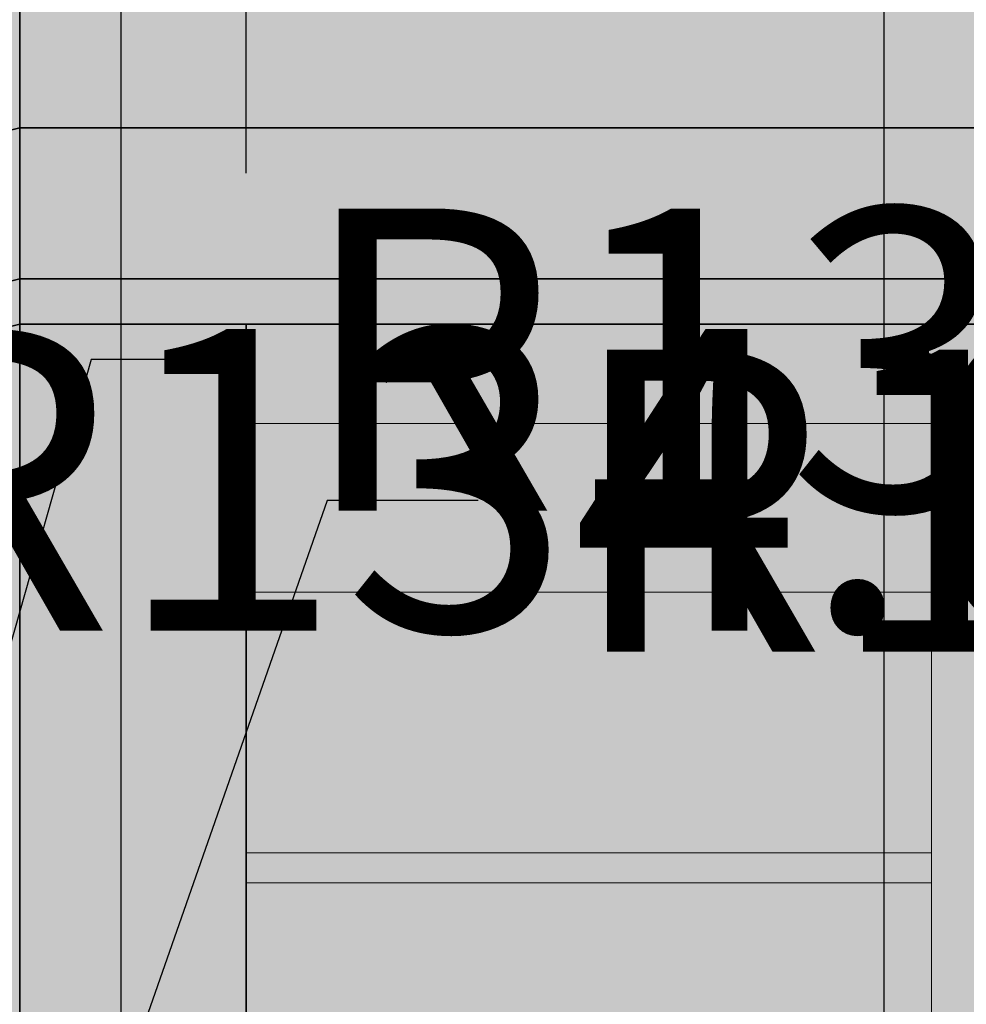
# Model space of a CAD drawing. Units: millimetres. Extents: x 130 to 1021, y 147 to 699.
# Tile 34 of 40: x 487 to 550, y 539 to 604. Entities that reach past the tile are written whole.
import ezdxf

# ---------------------------------------------------------------- set-up
doc = ezdxf.new("R2010")
doc.units = ezdxf.units.MM
doc.header["$MEASUREMENT"] = 0
for name, color, linetype, lineweight in [('A-ANNO-DIMS', 2, 'Continuous', 18), ('A-ELEV', 7, 'Continuous', 35), ('A-ELEV-PATT', 9, 'Continuous', 13), ('A-GLAZ', 4, 'Continuous', 18)]:
    doc.layers.add(name, color=color, linetype=linetype, lineweight=lineweight)
doc.styles.get("Standard").update_dxf_attribs({"font": 'arial.ttf'})
doc.dimstyles.get("Standard").update_dxf_attribs({"dimtxt": 20, "dimasz": 10, "dimexe": 10, "dimexo": 10, "dimgap": 5, "dimtad": 0, "dimtih": 1, "dimtoh": 1, "dimdec": 0, "dimzin": 0, "dimdsep": 46, "dimtxsty": 'Standard', "dimcen": 5, "dimadec": 0, "dimazin": 0, "dimtfac": 1, "dimtdec": 0, "dimtofl": 0, "dimtmove": 0, "dimatfit": 3, "dimfxl": 1, "dimtolj": 1, "dimtzin": 0, "dimarcsym": 0})

# ---------------------------------------------------------------- blocks, each defined once
blk = doc.blocks.new('*D11')
at = {"layer": 'A-ANNO-DIMS', "color": 0, "lineweight": -2, "transparency": 16777216}
for p, q in [((737.374, 648.699), (737.374, 149.739)), ((299.374, 566.947), (299.374, 149.739)), ((309.374, 159.739), (490.857, 159.739)), ((727.374, 159.739), (545.891, 159.739))]:
    blk.add_line(p, q, dxfattribs=at)
at = {"layer": 'A-ANNO-DIMS', "color": 0, "transparency": 16777216}
for points in [[(309.374, 161.406), (309.374, 158.073), (299.374, 159.739)], [(727.374, 161.406), (727.374, 158.073), (737.374, 159.739)]]:
    blk.add_solid(points, dxfattribs=at)
at = {"layer": 'Defpoints', "color": 0, "transparency": 16777216}
for p in [(737.374, 658.699), (299.374, 576.947), (737.374, 159.739)]:
    blk.add_point(p, dxfattribs=at)
at = {"layer": 'A-ANNO-DIMS', "color": 0, "transparency": 16777216, "insert": (518.374, 159.739), "char_height": 20, "attachment_point": 5}
blk.add_mtext('\\A1;438', dxfattribs=at)
blk = doc.blocks.new('*D12')
at = {"layer": 'A-ANNO-DIMS', "color": 0, "lineweight": -2, "transparency": 16777216}
for p, q in [((477.374, 661.947), (265.074, 661.947)), ((275.074, 651.947), (275.074, 438.205)), ((275.074, 194.039), (275.074, 407.782)), ((357.163, 184.039), (265.074, 184.039))]:
    blk.add_line(p, q, dxfattribs=at)
at = {"layer": 'A-ANNO-DIMS', "color": 0, "transparency": 16777216}
for points in [[(273.407, 651.947), (276.74, 651.947), (275.074, 661.947)], [(273.407, 194.039), (276.74, 194.039), (275.074, 184.039)]]:
    blk.add_solid(points, dxfattribs=at)
at = {"layer": 'Defpoints', "color": 0, "transparency": 16777216}
for p in [(275.074, 661.947), (487.374, 661.947), (367.163, 184.039)]:
    blk.add_point(p, dxfattribs=at)
at = {"layer": 'A-ANNO-DIMS', "color": 0, "transparency": 16777216, "insert": (275.074, 422.993), "char_height": 20, "attachment_point": 5}
blk.add_mtext('\\A1;477.9', dxfattribs=at)
blk = doc.blocks.new('*D19')
at = {"layer": 'A-ANNO-DIMS', "color": 0, "lineweight": -2, "transparency": 16777216}
for p, q in [((382.374, 388.947), (382.374, 696.247)), ((414.652, 510.881), (414.652, 696.247)), ((392.374, 686.247), (404.652, 686.247)), ((414.652, 686.247), (424.652, 686.247))]:
    blk.add_line(p, q, dxfattribs=at)
at = {"layer": 'A-ANNO-DIMS', "color": 0, "transparency": 16777216}
for points in [[(392.374, 687.914), (392.374, 684.581), (382.374, 686.247)], [(404.652, 687.914), (404.652, 684.581), (414.652, 686.247)]]:
    blk.add_solid(points, dxfattribs=at)
at = {"layer": 'Defpoints', "color": 0, "transparency": 16777216}
for p in [(414.652, 686.247), (414.652, 500.881), (382.374, 378.947)]:
    blk.add_point(p, dxfattribs=at)
at = {"layer": 'A-ANNO-DIMS', "color": 0, "transparency": 16777216, "insert": (463.411, 686.247), "char_height": 20, "attachment_point": 5}
blk.add_mtext('\\A1;32.28', dxfattribs=at)
blk = doc.blocks.new('*D20')
at = {"layer": 'A-ANNO-DIMS', "color": 0, "lineweight": -2, "transparency": 16777216}
for p, q in [((414.652, 510.881), (414.652, 696.247)), ((432.374, 388.947), (432.374, 696.247)), ((404.652, 686.247), (394.652, 686.247)), ((442.374, 686.247), (452.374, 686.247))]:
    blk.add_line(p, q, dxfattribs=at)
at = {"layer": 'A-ANNO-DIMS', "color": 0, "transparency": 16777216}
for points in [[(404.652, 687.914), (404.652, 684.581), (414.652, 686.247)], [(442.374, 687.914), (442.374, 684.581), (432.374, 686.247)]]:
    blk.add_solid(points, dxfattribs=at)
at = {"layer": 'Defpoints', "color": 0, "transparency": 16777216}
for p in [(432.374, 686.247), (414.652, 500.881), (432.374, 378.947)]:
    blk.add_point(p, dxfattribs=at)
at = {"layer": 'A-ANNO-DIMS', "color": 0, "transparency": 16777216, "insert": (490.075, 686.247), "char_height": 20, "attachment_point": 5}
blk.add_mtext('\\A1;17.72', dxfattribs=at)
blk = doc.blocks.new('*D21')
at = {"layer": 'A-ANNO-DIMS', "color": 0, "lineweight": -2, "transparency": 16777216}
for p, q in [((432.374, 388.947), (432.374, 696.247)), ((447.374, 656.947), (447.374, 696.247)), ((422.374, 686.247), (412.374, 686.247)), ((457.374, 686.247), (467.374, 686.247))]:
    blk.add_line(p, q, dxfattribs=at)
at = {"layer": 'A-ANNO-DIMS', "color": 0, "transparency": 16777216}
for points in [[(422.374, 687.914), (422.374, 684.581), (432.374, 686.247)], [(457.374, 687.914), (457.374, 684.581), (447.374, 686.247)]]:
    blk.add_solid(points, dxfattribs=at)
at = {"layer": 'Defpoints', "color": 0, "transparency": 16777216}
for p in [(447.374, 686.247), (447.374, 646.947), (432.374, 378.947)]:
    blk.add_point(p, dxfattribs=at)
at = {"layer": 'A-ANNO-DIMS', "color": 0, "transparency": 16777216, "insert": (485.832, 686.247), "char_height": 20, "attachment_point": 5}
blk.add_mtext('\\A1;15', dxfattribs=at)
blk = doc.blocks.new('*D22')
at = {"layer": 'A-ANNO-DIMS', "color": 0, "lineweight": -2, "transparency": 16777216}
for p, q in [((447.374, 656.947), (447.374, 696.247)), ((466.767, 403.947), (466.767, 696.247)), ((437.374, 686.247), (427.374, 686.247)), ((476.767, 686.247), (486.767, 686.247))]:
    blk.add_line(p, q, dxfattribs=at)
at = {"layer": 'A-ANNO-DIMS', "color": 0, "transparency": 16777216}
for points in [[(437.374, 687.914), (437.374, 684.581), (447.374, 686.247)], [(476.767, 687.914), (476.767, 684.581), (466.767, 686.247)]]:
    blk.add_solid(points, dxfattribs=at)
at = {"layer": 'Defpoints', "color": 0, "transparency": 16777216}
for p in [(466.767, 686.247), (447.374, 646.947), (466.767, 393.947)]:
    blk.add_point(p, dxfattribs=at)
at = {"layer": 'A-ANNO-DIMS', "color": 0, "transparency": 16777216, "insert": (532.34, 686.247), "char_height": 20, "attachment_point": 5}
blk.add_mtext('\\A1;19.393', dxfattribs=at)
blk = doc.blocks.new('*D23')
at = {"layer": 'A-ANNO-DIMS', "color": 0, "lineweight": -2, "transparency": 16777216}
for p, q in [((466.767, 403.947), (466.767, 696.247)), ((475.988, 209.039), (475.988, 696.247)), ((456.767, 686.247), (446.767, 686.247)), ((485.988, 686.247), (495.988, 686.247))]:
    blk.add_line(p, q, dxfattribs=at)
at = {"layer": 'A-ANNO-DIMS', "color": 0, "transparency": 16777216}
for points in [[(456.767, 687.914), (456.767, 684.581), (466.767, 686.247)], [(485.988, 687.914), (485.988, 684.581), (475.988, 686.247)]]:
    blk.add_solid(points, dxfattribs=at)
at = {"layer": 'Defpoints', "color": 0, "transparency": 16777216}
for p in [(475.988, 686.247), (466.767, 393.947), (475.988, 199.039)]:
    blk.add_point(p, dxfattribs=at)
at = {"layer": 'A-ANNO-DIMS', "color": 0, "transparency": 16777216, "insert": (534.631, 686.247), "char_height": 20, "attachment_point": 5}
blk.add_mtext('\\A1;9.222', dxfattribs=at)
blk = doc.blocks.new('*D24')
at = {"layer": 'A-ANNO-DIMS', "color": 0, "lineweight": -2, "transparency": 16777216}
for p, q in [((475.988, 209.039), (475.988, 696.247)), ((487.374, 671.947), (487.374, 696.247)), ((465.988, 686.247), (455.988, 686.247)), ((497.374, 686.247), (507.374, 686.247))]:
    blk.add_line(p, q, dxfattribs=at)
at = {"layer": 'A-ANNO-DIMS', "color": 0, "transparency": 16777216}
for points in [[(465.988, 687.914), (465.988, 684.581), (475.988, 686.247)], [(497.374, 687.914), (497.374, 684.581), (487.374, 686.247)]]:
    blk.add_solid(points, dxfattribs=at)
at = {"layer": 'Defpoints', "color": 0, "transparency": 16777216}
for p in [(487.374, 686.247), (487.374, 661.947), (475.988, 199.039)]:
    blk.add_point(p, dxfattribs=at)
at = {"layer": 'A-ANNO-DIMS', "color": 0, "transparency": 16777216, "insert": (553.022, 686.247), "char_height": 20, "attachment_point": 5}
blk.add_mtext('\\A1;11.385', dxfattribs=at)
blk = doc.blocks.new('*D25')
at = {"layer": 'A-ANNO-DIMS', "color": 0, "lineweight": -2, "transparency": 16777216}
for p, q in [((487.374, 671.947), (487.374, 696.247)), ((494.102, 506.908), (494.102, 696.247)), ((477.374, 686.247), (467.374, 686.247)), ((504.102, 686.247), (514.102, 686.247))]:
    blk.add_line(p, q, dxfattribs=at)
at = {"layer": 'A-ANNO-DIMS', "color": 0, "transparency": 16777216}
for points in [[(477.374, 687.914), (477.374, 684.581), (487.374, 686.247)], [(504.102, 687.914), (504.102, 684.581), (494.102, 686.247)]]:
    blk.add_solid(points, dxfattribs=at)
at = {"layer": 'Defpoints', "color": 0, "transparency": 16777216}
for p in [(494.102, 686.247), (487.374, 661.947), (494.102, 496.908)]:
    blk.add_point(p, dxfattribs=at)
at = {"layer": 'A-ANNO-DIMS', "color": 0, "transparency": 16777216, "insert": (552.922, 686.247), "char_height": 20, "attachment_point": 5}
blk.add_mtext('\\A1;6.728', dxfattribs=at)
blk = doc.blocks.new('*D26')
at = {"layer": 'A-ANNO-DIMS', "color": 0, "lineweight": -2, "transparency": 16777216}
for p, q in [((494.102, 506.908), (494.102, 696.247)), ((502.374, 593.947), (502.374, 696.247)), ((484.102, 686.247), (474.102, 686.247)), ((512.374, 686.247), (522.374, 686.247))]:
    blk.add_line(p, q, dxfattribs=at)
at = {"layer": 'A-ANNO-DIMS', "color": 0, "transparency": 16777216}
for points in [[(484.102, 687.914), (484.102, 684.581), (494.102, 686.247)], [(512.374, 687.914), (512.374, 684.581), (502.374, 686.247)]]:
    blk.add_solid(points, dxfattribs=at)
at = {"layer": 'Defpoints', "color": 0, "transparency": 16777216}
for p in [(502.374, 686.247), (502.374, 583.947), (494.102, 496.908)]:
    blk.add_point(p, dxfattribs=at)
at = {"layer": 'A-ANNO-DIMS', "color": 0, "transparency": 16777216, "insert": (561.03, 686.247), "char_height": 20, "attachment_point": 5}
blk.add_mtext('\\A1;8.272', dxfattribs=at)
blk = doc.blocks.new('*D27')
at = {"layer": 'A-ANNO-DIMS', "color": 0, "lineweight": -2, "transparency": 16777216}
for p, q in [((502.374, 593.947), (502.374, 696.247)), ((544.635, 396.264), (544.635, 696.247)), ((512.374, 686.247), (534.635, 686.247)), ((544.635, 686.247), (554.635, 686.247))]:
    blk.add_line(p, q, dxfattribs=at)
at = {"layer": 'A-ANNO-DIMS', "color": 0, "transparency": 16777216}
for points in [[(512.374, 687.914), (512.374, 684.581), (502.374, 686.247)], [(534.635, 687.914), (534.635, 684.581), (544.635, 686.247)]]:
    blk.add_solid(points, dxfattribs=at)
at = {"layer": 'Defpoints', "color": 0, "transparency": 16777216}
for p in [(544.635, 686.247), (502.374, 583.947), (544.635, 386.264)]:
    blk.add_point(p, dxfattribs=at)
at = {"layer": 'A-ANNO-DIMS', "color": 0, "transparency": 16777216, "insert": (593.776, 686.247), "char_height": 20, "attachment_point": 5}
blk.add_mtext('\\A1;42.26', dxfattribs=at)
blk = doc.blocks.new('*D28')
at = {"layer": 'A-ANNO-DIMS', "color": 0, "lineweight": -2, "transparency": 16777216}
for p, q in [((544.635, 396.264), (544.635, 696.247)), ((552.374, 593.947), (552.374, 696.247)), ((534.635, 686.247), (524.635, 686.247)), ((562.374, 686.247), (572.374, 686.247))]:
    blk.add_line(p, q, dxfattribs=at)
at = {"layer": 'A-ANNO-DIMS', "color": 0, "transparency": 16777216}
for points in [[(534.635, 687.914), (534.635, 684.581), (544.635, 686.247)], [(562.374, 687.914), (562.374, 684.581), (552.374, 686.247)]]:
    blk.add_solid(points, dxfattribs=at)
at = {"layer": 'Defpoints', "color": 0, "transparency": 16777216}
for p in [(552.374, 686.247), (552.374, 583.947), (544.635, 386.264)]:
    blk.add_point(p, dxfattribs=at)
at = {"layer": 'A-ANNO-DIMS', "color": 0, "transparency": 16777216, "insert": (611.057, 686.247), "char_height": 20, "attachment_point": 5}
blk.add_mtext('\\A1;7.738', dxfattribs=at)
blk = doc.blocks.new('*D57')
at = {"layer": 'A-ANNO-DIMS', "color": 0, "lineweight": -2, "transparency": 16777216}
for p, q in [((761.674, 606.947), (761.674, 616.947)), ((761.674, 616.947), (771.674, 616.947)), ((497.374, 596.947), (771.674, 596.947)), ((562.374, 583.947), (771.674, 583.947)), ((761.674, 573.947), (761.674, 563.947))]:
    blk.add_line(p, q, dxfattribs=at)
at = {"layer": 'A-ANNO-DIMS', "color": 0, "transparency": 16777216}
for points in [[(760.007, 606.947), (763.34, 606.947), (761.674, 596.947)], [(760.007, 573.947), (763.34, 573.947), (761.674, 583.947)]]:
    blk.add_solid(points, dxfattribs=at)
at = {"layer": 'Defpoints', "color": 0, "transparency": 16777216}
for p in [(487.374, 596.947), (761.674, 596.947), (552.374, 583.947)]:
    blk.add_point(p, dxfattribs=at)
at = {"layer": 'A-ANNO-DIMS', "color": 0, "transparency": 16777216, "insert": (790.057, 616.947), "char_height": 20, "attachment_point": 5}
blk.add_mtext('\\A1;13', dxfattribs=at)
blk = doc.blocks.new('*D58')
at = {"layer": 'A-ANNO-DIMS', "color": 0, "lineweight": -2, "transparency": 16777216}
for p, q in [((761.674, 656.947), (761.674, 666.947)), ((497.374, 646.947), (771.674, 646.947)), ((497.374, 596.947), (771.674, 596.947)), ((761.674, 586.947), (761.674, 576.947))]:
    blk.add_line(p, q, dxfattribs=at)
at = {"layer": 'A-ANNO-DIMS', "color": 0, "transparency": 16777216}
for points in [[(760.007, 656.947), (763.34, 656.947), (761.674, 646.947)], [(760.007, 586.947), (763.34, 586.947), (761.674, 596.947)]]:
    blk.add_solid(points, dxfattribs=at)
at = {"layer": 'Defpoints', "color": 0, "transparency": 16777216}
for p in [(487.374, 646.947), (761.674, 646.947), (487.374, 596.947)]:
    blk.add_point(p, dxfattribs=at)
at = {"layer": 'A-ANNO-DIMS', "color": 0, "transparency": 16777216, "insert": (761.674, 621.947), "char_height": 20, "attachment_point": 5}
blk.add_mtext('\\A1;50', dxfattribs=at)
blk = doc.blocks.new('*D69')
at = {"layer": 'A-ANNO-DIMS', "color": 0, "lineweight": -2, "transparency": 16777216}
for p, q in [((507.746, 572.261), (483.091, 501.813)), ((517.746, 572.261), (507.746, 572.261)), ((433.191, 354.23), (433.191, 364.23)), ((428.191, 359.23), (438.191, 359.23))]:
    blk.add_line(p, q, dxfattribs=at)
at = {"layer": 'A-ANNO-DIMS', "color": 0, "transparency": 16777216}
blk.add_solid([(481.518, 502.363), (484.664, 501.262), (479.788, 492.374)], dxfattribs=at)
at = {"layer": 'Defpoints', "color": 0, "transparency": 16777216}
for p in [(479.788, 492.374), (433.191, 359.23)]:
    blk.add_point(p, dxfattribs=at)
at = {"layer": 'A-ANNO-DIMS', "color": 0, "transparency": 16777216, "insert": (573.824, 572.261), "char_height": 20, "attachment_point": 5}
blk.add_mtext('\\A1;R141.06', dxfattribs=at)
blk = doc.blocks.new('*D71')
at = {"layer": 'A-ANNO-DIMS', "color": 0, "lineweight": -2, "transparency": 16777216}
for p, q in [((492.108, 581.609), (472.542, 512.666)), ((502.108, 581.609), (492.108, 581.609)), ((432.65, 367.109), (432.65, 377.109)), ((427.65, 372.109), (437.65, 372.109))]:
    blk.add_line(p, q, dxfattribs=at)
at = {"layer": 'A-ANNO-DIMS', "color": 0, "transparency": 16777216}
blk.add_solid([(470.938, 513.121), (474.145, 512.211), (469.812, 503.046)], dxfattribs=at)
at = {"layer": 'Defpoints', "color": 0, "transparency": 16777216}
for p in [(469.812, 503.046), (432.65, 372.109)]:
    blk.add_point(p, dxfattribs=at)
at = {"layer": 'A-ANNO-DIMS', "color": 0, "transparency": 16777216, "insert": (548.493, 581.609), "char_height": 20, "attachment_point": 5}
blk.add_mtext('\\A1;R136.1', dxfattribs=at)
blk = doc.blocks.new('*D72')
at = {"layer": 'A-ANNO-DIMS', "color": 0, "lineweight": -2, "transparency": 16777216}
for p, q in [((460.658, 573.64), (451.279, 503.49)), ((470.658, 573.64), (460.658, 573.64)), ((432.115, 355.142), (432.115, 365.142)), ((427.115, 360.142), (437.115, 360.142))]:
    blk.add_line(p, q, dxfattribs=at)
at = {"layer": 'A-ANNO-DIMS', "color": 0, "transparency": 16777216}
blk.add_solid([(449.628, 503.711), (452.931, 503.27), (449.954, 493.579)], dxfattribs=at)
at = {"layer": 'Defpoints', "color": 0, "transparency": 16777216}
for p in [(449.954, 493.579), (432.115, 360.142)]:
    blk.add_point(p, dxfattribs=at)
at = {"layer": 'A-ANNO-DIMS', "color": 0, "transparency": 16777216, "insert": (526.64, 573.64), "char_height": 20, "attachment_point": 5}
blk.add_mtext('\\A1;R134.62', dxfattribs=at)

msp = doc.modelspace()

# ---------------------------------------------------------------- hatches: boundary and pattern name
at = {"layer": 'A-ELEV-PATT'}
h = msp.add_hatch(color=256, dxfattribs=at)
h.dxf.hatch_style = 1
h.paths.add_polyline_path([(737.3738, 658.6988, 0.0135961), (632.4019, 661.9473), (607.3738, 661.9473), (487.3738, 661.9473), (487.3738, 649.9473), (607.3738, 649.9473), (632.3794, 649.9473, -0.0136841), (737.3738, 646.6784)])
h.paths.add_polyline_path([(732.3738, 643.9599, 0.0130529), (632.3738, 646.9473), (607.3738, 646.9473), (487.3738, 646.9473), (487.3738, 596.9473), (632.3738, 596.9473, -0.0130529), (732.3738, 593.9599)])
h.paths.add_polyline_path([(737.3738, 593.6732, 0.0137063), (632.3738, 596.9473), (487.3738, 596.9473), (487.3738, 586.9473), (632.355, 586.9473, -0.0137808), (737.3738, 583.6559)])
h.paths.add_polyline_path([(447.3738, 646.9473), (307.3738, 646.9473), (302.3738, 646.9473), (302.3738, 634.9473), (447.3738, 634.9473)])
h.paths.add_polyline_path([(447.3738, 631.9473), (307.3738, 631.9473), (307.3738, 586.9473), (447.3738, 586.9473)])
h.paths.add_polyline_path([(447.3738, 586.9473), (307.3738, 586.9473), (302.3738, 586.9473), (302.3738, 576.9473), (447.3738, 576.9473)])
h.paths.add_polyline_path([(447.3738, 573.9473), (367.3738, 573.9473), (367.3738, 539.9473), (447.3738, 539.9473)])
h.paths.add_polyline_path([(447.3738, 537.9473), (367.3738, 537.9473), (367.3738, 507.9473), (400.392, 507.4253, -0.001728), (401.3281, 507.6451, -0.5220025), (425.6117, 511.0391, -0.0391849), (447.3738, 510.4359), (447.3738, 510.7883)])
h.paths.add_polyline_path([(394.7238, 505.9473), (367.3738, 505.9473), (367.3738, 476.9473, -0.0146512), (375.8501, 480.2159), (376.1506, 499.2266, -0.0355419)])
h.paths.add_polyline_path([(632.3738, 583.9473), (552.3738, 583.9473), (552.3738, 550.9473), (632.3738, 550.9473)])
h.paths.add_polyline_path([(632.3738, 548.9473), (552.3738, 548.9473), (552.3738, 515.9473), (632.3738, 515.9473)])
h.paths.add_polyline_path([(632.3738, 513.9473), (552.3738, 513.9473), (552.3738, 476.9473), (632.3738, 476.9473)])
h.paths.add_polyline_path([(737.3738, 473.6903, 0.0136326), (632.3926, 476.9473), (552.3738, 476.9473), (487.3738, 476.9473), (487.3738, 466.9473), (632.3738, 466.9473, -0.0137063), (737.3738, 463.6732)])
h.paths.add_polyline_path([(732.3738, 460.9552, 0.0130741), (632.3681, 463.9473), (487.3738, 463.9473), (487.3738, 407.735, -0.0032286), (489.3544, 406.9473), (632.3926, 406.9473, -0.0129826), (732.3738, 403.9755)])
h.paths.add_polyline_path([(487.3738, 463.9473, 0.20133), (367.3738, 463.9473), (367.3738, 407.735, -0.1882031), (487.3738, 407.735)])
h.paths.add_polyline_path([(367.3738, 476.9473), (367.3738, 466.9473, -0.2013309), (487.3738, 466.9473), (487.3738, 476.9473, 0.20133)])
h.paths.add_polyline_path([(367.3738, 463.9473), (307.3738, 463.9473), (307.3738, 401.9473), (357.9413, 401.9473), (367.3738, 407.735)])
h.paths.add_polyline_path([(367.3738, 476.9473), (302.3738, 476.9473), (302.3738, 466.9473), (367.3738, 466.9473)])
h.paths.add_polyline_path([(632.8184, 366.9453), (552.3738, 366.9453), (552.3738, 393.9473), (632.8184, 393.9473)])
h.paths.add_polyline_path([(632.8184, 357.2114), (632.8184, 363.9453), (552.3738, 363.9453), (552.3738, 357.2114), (552.3738, 336.9453), (632.8184, 336.9453)])
h.paths.add_polyline_path([(632.8184, 333.9453), (552.3738, 333.9453), (552.3738, 306.9453), (632.8184, 306.9453)])
h.paths.add_polyline_path([(632.8184, 303.9453), (552.3738, 303.9453), (552.3738, 273.9473), (632.355, 273.9473, 0.0000608), (632.8184, 273.9491)])
h.paths.add_polyline_path([(737.3738, 403.6903, 0.0136326), (632.3926, 406.9473), (489.3544, 406.9473, 0.1915481), (367.3738, 407.735), (367.3738, 396.9473, -0.2013309), (487.3738, 396.9473), (632.3738, 396.9473, -0.0137063), (737.3738, 393.6732)])
h.paths.add_polyline_path([(357.9413, 401.9473), (307.3738, 401.9473), (307.3738, 391.9473), (357.9413, 391.9473)])
h.paths.add_polyline_path([(357.9413, 357.2114), (357.9413, 388.9473), (307.3738, 388.9473), (307.3738, 357.2114), (307.3738, 273.9473), (357.9413, 273.9473)])
h.paths.add_polyline_path([(732.3738, 263.93, -0.0130317), (632.3794, 260.9473), (466.7667, 260.9473), (466.7667, 240.9473), (469.8406, 236.978), (469.8406, 221.978), (472.9145, 218.0087), (472.9145, 213.9473), (607.3738, 213.9473), (732.3738, 213.9473)])
h.paths.add_polyline_path([(732.3738, 290.889), (722.479, 290.889), (722.479, 301.889), (732.3738, 301.889), (732.3738, 305.889), (722.479, 305.889), (722.479, 316.889), (732.3738, 316.889), (732.3738, 320.889), (722.479, 320.889), (722.479, 331.889), (732.3738, 331.889), (732.3738, 335.889), (722.479, 335.889), (722.479, 346.889), (732.3738, 346.889), (732.3738, 350.889), (722.479, 350.889), (722.479, 361.889), (732.3738, 361.889), (732.3738, 365.889), (722.479, 365.889), (722.479, 376.889), (732.3738, 376.889), (732.3738, 380.889), (722.479, 380.889), (722.479, 391.4848, 0.0005233), (718.479, 391.6843), (718.479, 380.889), (707.479, 380.889), (707.479, 392.1896, 0.0005231), (703.479, 392.3576), (703.479, 380.889), (692.479, 380.889), (692.479, 392.7765, 0.0005229), (688.479, 392.9131), (688.479, 380.889), (677.479, 380.889), (677.479, 393.2456, 0.0005228), (673.479, 393.3508), (673.479, 380.889), (662.479, 380.889), (662.479, 393.597, 0.0005227), (658.479, 393.6709), (658.479, 380.889), (647.479, 380.889), (647.479, 393.8308, 0.0005226), (643.479, 393.8732), (643.479, 380.889), (632.8184, 380.889), (632.8184, 376.889), (643.479, 376.889), (643.479, 365.889), (632.8184, 365.889), (632.8184, 361.889), (643.479, 361.889), (643.479, 350.889), (632.8184, 350.889), (632.8184, 346.889), (643.479, 346.889), (643.479, 335.889), (632.8184, 335.889), (632.8184, 331.889), (643.479, 331.889), (643.479, 320.889), (632.8184, 320.889), (632.8184, 316.889), (643.479, 316.889), (643.479, 305.889), (632.8184, 305.889), (632.8184, 301.889), (643.479, 301.889), (643.479, 290.889), (632.8184, 290.889), (632.8184, 286.889), (643.479, 286.889), (643.479, 274.0217, 0.0005246), (647.479, 274.0643), (647.479, 286.889), (658.479, 286.889), (658.479, 274.2248, 0.0005246), (662.479, 274.2989), (662.479, 286.889), (673.479, 286.889), (673.479, 274.546, 0.0005247), (677.479, 274.6516), (677.479, 286.889), (688.479, 286.889), (688.479, 274.9853, 0.0005248), (692.479, 275.1224), (692.479, 286.889), (703.479, 286.889), (703.479, 275.5429, 0.000525), (707.479, 275.7115), (707.479, 286.889), (718.479, 286.889), (718.479, 276.2187, 0.0005252), (722.479, 276.4189), (722.479, 286.889), (732.3738, 286.889)])
h.paths.add_polyline_path([(718.479, 290.889), (707.479, 290.889), (707.479, 301.889), (718.479, 301.889)], flags=16)
h.paths.add_polyline_path([(703.479, 290.889), (692.479, 290.889), (692.479, 301.889), (703.479, 301.889)], flags=16)
h.paths.add_polyline_path([(718.479, 305.889), (707.479, 305.889), (707.479, 316.889), (718.479, 316.889)], flags=16)
h.paths.add_polyline_path([(703.479, 305.889), (692.479, 305.889), (692.479, 316.889), (703.479, 316.889)], flags=16)
h.paths.add_polyline_path([(688.479, 290.889), (677.479, 290.889), (677.479, 301.889), (688.479, 301.889)], flags=16)
h.paths.add_polyline_path([(718.479, 320.889), (707.479, 320.889), (707.479, 331.889), (718.479, 331.889)], flags=16)
h.paths.add_polyline_path([(688.479, 305.889), (677.479, 305.889), (677.479, 316.889), (688.479, 316.889)], flags=16)
h.paths.add_polyline_path([(703.479, 320.889), (692.479, 320.889), (692.479, 331.889), (703.479, 331.889)], flags=16)
h.paths.add_polyline_path([(688.479, 320.889), (677.479, 320.889), (677.479, 331.889), (688.479, 331.889)], flags=16)
h.paths.add_polyline_path([(673.479, 290.889), (662.479, 290.889), (662.479, 301.889), (673.479, 301.889)], flags=16)
h.paths.add_polyline_path([(718.479, 335.889), (707.479, 335.889), (707.479, 346.889), (718.479, 346.889)], flags=16)
h.paths.add_polyline_path([(673.479, 305.889), (662.479, 305.889), (662.479, 316.889), (673.479, 316.889)], flags=16)
h.paths.add_polyline_path([(703.479, 335.889), (692.479, 335.889), (692.479, 346.889), (703.479, 346.889)], flags=16)
h.paths.add_polyline_path([(673.479, 320.889), (662.479, 320.889), (662.479, 331.889), (673.479, 331.889)], flags=16)
h.paths.add_polyline_path([(688.479, 335.889), (677.479, 335.889), (677.479, 346.889), (688.479, 346.889)], flags=16)
h.paths.add_polyline_path([(658.479, 290.889), (647.479, 290.889), (647.479, 301.889), (658.479, 301.889)], flags=16)
h.paths.add_polyline_path([(718.479, 350.889), (707.479, 350.889), (707.479, 361.889), (718.479, 361.889)], flags=16)
h.paths.add_polyline_path([(658.479, 305.889), (647.479, 305.889), (647.479, 316.889), (658.479, 316.889)], flags=16)
h.paths.add_polyline_path([(703.479, 350.889), (692.479, 350.889), (692.479, 361.889), (703.479, 361.889)], flags=16)
h.paths.add_polyline_path([(673.479, 335.889), (662.479, 335.889), (662.479, 346.889), (673.479, 346.889)], flags=16)
h.paths.add_polyline_path([(658.479, 320.889), (647.479, 320.889), (647.479, 331.889), (658.479, 331.889)], flags=16)
h.paths.add_polyline_path([(688.479, 350.889), (677.479, 350.889), (677.479, 361.889), (688.479, 361.889)], flags=16)
h.paths.add_polyline_path([(718.479, 365.889), (707.479, 365.889), (707.479, 376.889), (718.479, 376.889)], flags=16)
h.paths.add_polyline_path([(658.479, 335.889), (647.479, 335.889), (647.479, 346.889), (658.479, 346.889)], flags=16)
h.paths.add_polyline_path([(673.479, 350.889), (662.479, 350.889), (662.479, 361.889), (673.479, 361.889)], flags=16)
h.paths.add_polyline_path([(703.479, 365.889), (692.479, 365.889), (692.479, 376.889), (703.479, 376.889)], flags=16)
h.paths.add_polyline_path([(688.479, 365.889), (677.479, 365.889), (677.479, 376.889), (688.479, 376.889)], flags=16)
h.paths.add_polyline_path([(658.479, 350.889), (647.479, 350.889), (647.479, 361.889), (658.479, 361.889)], flags=16)
h.paths.add_polyline_path([(673.479, 365.889), (662.479, 365.889), (662.479, 376.889), (673.479, 376.889)], flags=16)
h.paths.add_polyline_path([(658.479, 365.889), (647.479, 365.889), (647.479, 376.889), (658.479, 376.889)], flags=16)
h.paths.add_polyline_path([(732.3738, 503.9786), (722.3392, 503.9786), (722.3392, 514.9786), (732.3738, 514.9786), (732.3738, 518.9786), (722.3392, 518.9786), (722.3392, 529.9786), (732.3738, 529.9786), (732.3738, 533.9786), (722.3392, 533.9786), (722.3392, 544.9786), (732.3738, 544.9786), (732.3738, 546.9473), (732.3738, 548.9786), (722.3392, 548.9786), (722.3392, 559.9786), (732.3738, 559.9786), (732.3738, 563.9786), (722.3392, 563.9786), (722.3392, 574.9786), (732.3738, 574.9786), (732.3738, 578.9786), (722.3392, 578.9786), (722.3392, 581.4789, 0.000526), (718.3392, 581.6791), (718.3392, 578.9786), (707.3392, 578.9786), (707.3392, 582.1863, 0.0005258), (703.3392, 582.355), (703.3392, 578.9786), (692.3392, 578.9786), (692.3392, 582.7752, 0.0005257), (688.3392, 582.9123), (688.3392, 578.9786), (677.3392, 578.9786), (677.3392, 583.2457, 0.0005255), (673.3392, 583.3512), (673.3392, 578.9786), (662.3392, 578.9786), (662.3392, 583.5978, 0.0005254), (658.3392, 583.6718), (658.3392, 578.9786), (647.3392, 578.9786), (647.3392, 583.8317, 0.0005254), (643.3392, 583.8741), (643.3392, 578.9786), (632.3738, 578.9786), (632.3738, 574.9786), (643.3392, 574.9786), (643.3392, 563.9786), (632.3738, 563.9786), (632.3738, 559.9786), (643.3392, 559.9786), (643.3392, 548.9786), (632.3738, 548.9786), (632.3738, 544.9786), (643.3392, 544.9786), (643.3392, 533.9786), (632.3738, 533.9786), (632.3738, 529.9786), (643.3392, 529.9786), (643.3392, 518.9786), (632.3738, 518.9786), (632.3738, 515.9473), (632.3738, 514.9786), (643.3392, 514.9786), (643.3392, 503.9786), (632.3738, 503.9786), (632.3738, 499.9786), (643.3392, 499.9786), (643.3392, 488.9786), (632.3738, 488.9786), (632.3738, 484.9786), (643.3392, 484.9786), (643.3392, 476.8751, -0.0005191), (647.3392, 476.8332), (647.3392, 484.9786), (658.3392, 484.9786), (658.3392, 476.6752, -0.0005192), (662.3392, 476.6022), (662.3392, 484.9786), (673.3392, 484.9786), (673.3392, 476.3585, -0.0005193), (677.3392, 476.2543), (677.3392, 484.9786), (688.3392, 484.9786), (688.3392, 475.9248, -0.0005194), (692.3392, 475.7894), (692.3392, 484.9786), (703.3392, 484.9786), (703.3392, 475.3741, -0.0005195), (707.3392, 475.2075), (707.3392, 484.9786), (718.3392, 484.9786), (718.3392, 474.7064, -0.0005197), (722.3392, 474.5086), (722.3392, 484.9786), (732.3738, 484.9786), (732.3738, 488.9786), (722.3392, 488.9786), (722.3392, 499.9786), (732.3738, 499.9786)])
h.paths.add_polyline_path([(718.3392, 503.9786), (707.3392, 503.9786), (707.3392, 514.9786), (718.3392, 514.9786)], flags=16)
h.paths.add_polyline_path([(718.3392, 499.9786), (718.3392, 488.9786), (707.3392, 488.9786), (707.3392, 499.9786)], flags=16)
h.paths.add_polyline_path([(718.3392, 518.9786), (707.3392, 518.9786), (707.3392, 529.9786), (718.3392, 529.9786)], flags=16)
h.paths.add_polyline_path([(703.3392, 503.9786), (692.3392, 503.9786), (692.3392, 514.9786), (703.3392, 514.9786)], flags=16)
h.paths.add_polyline_path([(703.3392, 499.9786), (703.3392, 488.9786), (692.3392, 488.9786), (692.3392, 499.9786)], flags=16)
h.paths.add_polyline_path([(703.3392, 518.9786), (692.3392, 518.9786), (692.3392, 529.9786), (703.3392, 529.9786)], flags=16)
h.paths.add_polyline_path([(718.3392, 533.9786), (707.3392, 533.9786), (707.3392, 544.9786), (718.3392, 544.9786)], flags=16)
h.paths.add_polyline_path([(688.3392, 503.9786), (677.3392, 503.9786), (677.3392, 514.9786), (688.3392, 514.9786)], flags=16)
h.paths.add_polyline_path([(688.3392, 499.9786), (688.3392, 488.9786), (677.3392, 488.9786), (677.3392, 499.9786)], flags=16)
h.paths.add_polyline_path([(703.3392, 533.9786), (692.3392, 533.9786), (692.3392, 544.9786), (703.3392, 544.9786)], flags=16)
h.paths.add_polyline_path([(688.3392, 518.9786), (677.3392, 518.9786), (677.3392, 529.9786), (688.3392, 529.9786)], flags=16)
h.paths.add_polyline_path([(688.3392, 533.9786), (677.3392, 533.9786), (677.3392, 544.9786), (688.3392, 544.9786)], flags=16)
h.paths.add_polyline_path([(718.3392, 548.9786), (707.3392, 548.9786), (707.3392, 559.9786), (718.3392, 559.9786)], flags=16)
h.paths.add_polyline_path([(673.3392, 503.9786), (662.3392, 503.9786), (662.3392, 514.9786), (673.3392, 514.9786)], flags=16)
h.paths.add_polyline_path([(673.3392, 499.9786), (673.3392, 488.9786), (662.3392, 488.9786), (662.3392, 499.9786)], flags=16)
h.paths.add_polyline_path([(703.3392, 548.9786), (692.3392, 548.9786), (692.3392, 559.9786), (703.3392, 559.9786)], flags=16)
h.paths.add_polyline_path([(673.3392, 518.9786), (662.3392, 518.9786), (662.3392, 529.9786), (673.3392, 529.9786)], flags=16)
h.paths.add_polyline_path([(688.3392, 548.9786), (677.3392, 548.9786), (677.3392, 559.9786), (688.3392, 559.9786)], flags=16)
h.paths.add_polyline_path([(673.3392, 533.9786), (662.3392, 533.9786), (662.3392, 544.9786), (673.3392, 544.9786)], flags=16)
h.paths.add_polyline_path([(718.3392, 563.9786), (707.3392, 563.9786), (707.3392, 574.9786), (718.3392, 574.9786)], flags=16)
h.paths.add_polyline_path([(658.3392, 503.9786), (647.3392, 503.9786), (647.3392, 514.9786), (658.3392, 514.9786)], flags=16)
h.paths.add_polyline_path([(658.3392, 499.9786), (658.3392, 488.9786), (647.3392, 488.9786), (647.3392, 499.9786)], flags=16)
h.paths.add_polyline_path([(703.3392, 563.9786), (692.3392, 563.9786), (692.3392, 574.9786), (703.3392, 574.9786)], flags=16)
h.paths.add_polyline_path([(658.3392, 518.9786), (647.3392, 518.9786), (647.3392, 529.9786), (658.3392, 529.9786)], flags=16)
h.paths.add_polyline_path([(673.3392, 548.9786), (662.3392, 548.9786), (662.3392, 559.9786), (673.3392, 559.9786)], flags=16)
h.paths.add_polyline_path([(688.3392, 563.9786), (677.3392, 563.9786), (677.3392, 574.9786), (688.3392, 574.9786)], flags=16)
h.paths.add_polyline_path([(658.3392, 533.9786), (647.3392, 533.9786), (647.3392, 544.9786), (658.3392, 544.9786)], flags=16)
h.paths.add_polyline_path([(673.3392, 563.9786), (662.3392, 563.9786), (662.3392, 574.9786), (673.3392, 574.9786)], flags=16)
h.paths.add_polyline_path([(658.3392, 548.9786), (647.3392, 548.9786), (647.3392, 559.9786), (658.3392, 559.9786)], flags=16)
h.paths.add_polyline_path([(658.3392, 563.9786), (647.3392, 563.9786), (647.3392, 574.9786), (658.3392, 574.9786)], flags=16)
h = msp.add_hatch(color=256, dxfattribs=at)
h.dxf.hatch_style = 1
h.paths.add_polyline_path([(487.3738, 649.9473), (487.3738, 661.9473), (447.3738, 646.9473), (447.3738, 634.9473)])
h.paths.add_polyline_path([(487.3738, 646.9473), (447.3738, 631.9473), (447.3738, 586.9473), (487.3738, 596.9473)])
h.paths.add_polyline_path([(487.3738, 596.9473), (447.3738, 586.9473), (447.3738, 576.9473), (487.3738, 586.9473)])
h.paths.add_polyline_path([(460.3738, 577.1973), (447.3738, 573.9473), (447.3738, 510.7883), (447.3738, 510.4359, -0.0236536), (460.3738, 508.4268), (460.3738, 509.3636)])
h.paths.add_polyline_path([(472.3738, 580.1973), (460.3738, 577.1973), (460.3738, 509.3636), (460.3738, 508.4268, -0.0055147), (463.3738, 507.7821), (463.3738, 508.8807), (463.3738, 572.7934), (469.3738, 574.2934), (469.3738, 507.7378), (469.3738, 506.2825, -0.0056075), (472.3738, 505.4251), (472.3738, 507.0765)])
h = msp.add_hatch(color=256, dxfattribs=at)
h.dxf.hatch_style = 1
h.paths.add_polyline_path([(447.3738, 576.9473), (302.3738, 576.9473), (302.3738, 573.9473), (447.3738, 573.9473)])
h.paths.add_polyline_path([(487.3738, 583.9473), (487.3738, 586.9473), (447.3738, 576.9473), (447.3738, 573.9473)])
h.paths.add_polyline_path([(632.355, 586.9473), (487.3738, 586.9473), (487.3738, 583.9473), (632.3738, 583.9473), (632.3738, 583.9472, -0.0138), (737.3738, 580.6507), (737.3738, 583.6559, 0.0137808)])
h.paths.add_polyline_path([(367.3738, 466.9473), (302.3738, 466.9473), (302.3738, 463.9473), (367.3738, 463.9473)])
h.paths.add_polyline_path([(487.3738, 463.9473), (487.3738, 466.9473, 0.2013309), (367.3738, 466.9473), (367.3738, 463.9473, -0.20133)])
h.paths.add_polyline_path([(632.3738, 466.9473), (487.3738, 466.9473), (487.3738, 463.9473), (632.3681, 463.9473, -0.0137285), (737.3738, 460.6681), (737.3738, 463.6732, 0.0137063)])
h.paths.add_polyline_path([(632.3738, 396.9473), (487.3738, 396.9473, 0.2013309), (367.3738, 396.9473), (367.3738, 393.9473, -0.2023717), (486.7667, 393.9473), (632.3681, 393.9473, -0.0137285), (737.3738, 390.6681), (737.3738, 393.6732, 0.0137063)])
h.paths.add_polyline_path([(357.9413, 391.9473), (307.3738, 391.9473), (307.3738, 388.9473), (357.9413, 388.9473)])
h.paths.add_polyline_path([(367.3738, 393.9473), (367.3738, 396.9473), (357.9413, 391.924), (357.9413, 388.9473), (358.058, 388.9473)])
h.paths.add_polyline_path([(737.3738, 264.2162), (737.3738, 267.2214, -0.0137063), (632.3738, 263.9473), (463.7667, 263.9473), (466.7667, 260.9473), (632.3794, 260.9473, 0.0136841)])
h.paths.add_polyline_path([(463.7667, 263.9473), (447.3738, 263.9473), (450.3738, 260.9473), (466.7667, 260.9473)])
h.paths.add_polyline_path([(447.3738, 263.9473), (432.3738, 263.9473), (432.3738, 260.9473), (450.3738, 260.9473)])
h.paths.add_polyline_path([(382.3738, 263.9473), (357.9413, 263.9473), (357.9413, 260.9473), (382.3738, 260.9473)])
h.paths.add_polyline_path([(357.9413, 263.9473), (307.3738, 263.9473), (307.3738, 260.9473), (357.9413, 260.9473)])
h = msp.add_hatch(color=256, dxfattribs=at)
h.paths.add_polyline_path([(327.3738, 569.884), (327.3738, 573.9473), (307.3738, 573.9473), (307.3738, 476.9473), (327.3738, 476.9473), (327.3738, 480.95)])
h.paths.add_polyline_path([(486.7667, 386.2639), (486.7667, 393.9473), (466.7667, 393.9473), (466.7667, 357.2114), (466.7667, 311.9335, 0.0342703), (486.7667, 308.4637)])
h.paths.add_polyline_path([(486.7667, 308.4637, -0.0342703), (466.7667, 311.9335), (466.7667, 273.9473), (486.7667, 273.9473)])
h.paths.add_polyline_path([(389.3738, 351.5473), (396.7693, 351.5473, -0.007027), (393.8774, 354.5473), (389.3738, 354.5473), (389.3738, 359.5775, -0.0190302), (382.3738, 368.424), (382.3738, 249.5473), (432.3738, 249.5473), (432.3738, 325.067, -0.0057673), (429.3738, 326.709), (429.3738, 257.5473), (426.3738, 257.5473), (426.3738, 328.4428, -0.0059254), (423.3738, 330.272), (423.3738, 315.7473), (389.3738, 315.7473), (389.3738, 332.1473), (420.4552, 332.1473, -0.008951), (416.0768, 335.1473), (389.3738, 335.1473)])
h.paths.add_polyline_path([(389.3738, 312.7473), (423.3738, 312.7473), (423.3738, 296.3473), (389.3738, 296.3473)], flags=16)
h.paths.add_polyline_path([(389.3738, 293.3473), (423.3738, 293.3473), (423.3738, 276.9473), (389.3738, 276.9473)], flags=16)
h.paths.add_polyline_path([(389.3738, 273.9473), (423.3738, 273.9473), (423.3738, 257.5473), (389.3738, 257.5473)], flags=16)
h.paths.add_polyline_path([(432.3738, 378.9473), (382.3738, 378.9473), (382.3738, 368.424, 0.0190302), (389.3738, 359.5775), (389.3738, 370.9473), (423.3738, 370.9473), (423.3738, 354.5473), (393.8774, 354.5473, 0.007027), (396.7693, 351.5473), (423.3738, 351.5473), (423.3738, 335.1473), (416.0768, 335.1473, 0.008951), (420.4552, 332.1473), (423.3738, 332.1473), (423.3738, 330.272, 0.0059254), (426.3738, 328.4428), (426.3738, 370.9473), (429.3738, 370.9473), (429.3738, 326.709, 0.0057673), (432.3738, 325.067)])
h.paths.add_polyline_path([(466.7667, 357.2114), (466.7667, 393.9473), (447.3738, 393.9473), (447.3738, 357.2114), (447.3738, 318.1243, 0.0063261), (450.8779, 316.785), (450.8779, 331.5915), (463.5608, 331.5915), (463.5608, 312.7571, 0.005582), (466.7667, 311.9335)])
h.paths.add_polyline_path([(450.8779, 334.5915), (450.8779, 360.0915), (463.5608, 360.0915), (463.5608, 334.5915)], flags=16)
h.paths.add_polyline_path([(450.8779, 363.0915), (450.8779, 388.6449), (463.5608, 388.6449), (463.5608, 363.0915)], flags=16)
h.paths.add_polyline_path([(466.7667, 311.9335, -0.005582), (463.5608, 312.7571), (463.5608, 306.0915), (450.8779, 306.0915), (450.8779, 316.785, -0.0063261), (447.3738, 318.1243), (447.3738, 273.9473), (466.7667, 273.9473)])
h.paths.add_polyline_path([(450.8779, 303.0915), (463.5608, 303.0915), (463.5608, 277.5915), (450.8779, 277.5915)], flags=16)
h.paths.add_polyline_path([(552.3738, 357.2114), (552.3738, 393.9473), (486.7667, 393.9473), (486.7667, 386.2639), (544.6354, 386.2639), (544.6354, 280.6619), (486.7667, 280.6619), (486.7667, 273.9473), (552.3738, 273.9473)])
h.paths.add_polyline_path([(487.3738, 583.9473), (472.3738, 580.1973), (472.3738, 507.0765), (472.3738, 505.4251, -0.0056452), (475.3738, 504.4942), (475.3738, 506.3543), (475.3738, 511.9473), (484.3738, 511.9473), (484.3738, 503.8134), (484.3738, 501.2439, -0.0058357), (487.3738, 500.0015)])
h.paths.add_polyline_path([(484.3738, 578.0434), (484.3738, 548.9473), (475.3738, 548.9473), (475.3738, 575.7934)], flags=16)
h.paths.add_polyline_path([(484.3738, 546.9473), (484.3738, 513.9473), (475.3738, 513.9473), (475.3738, 518.7148), (475.3738, 546.9473)], flags=16)
for points in [[(502.3738, 583.9473), (487.3738, 583.9473), (487.3738, 500.0015, -0.0133113), (494.1023, 496.908), (494.1023, 476.9473), (502.3738, 476.9473)], [(502.3738, 583.9473), (502.3738, 577.3739), (547.7773, 577.3739), (547.7773, 481.7432), (502.3738, 481.7432), (502.3738, 476.9473), (552.3738, 476.9473), (552.3738, 583.9473)]]:
    msp.add_hatch(color=256, dxfattribs=at).paths.add_polyline_path(points)
h = msp.add_hatch(color=256, dxfattribs=at)
h.dxf.hatch_style = 1
h.paths.add_polyline_path([(363.922, 569.884), (327.3738, 569.884), (327.3738, 557.9168), (363.922, 557.9168)])
h.paths.add_polyline_path([(547.7773, 577.3739), (502.3738, 577.3739), (502.3738, 566.2111), (547.7773, 566.2111)])
h.paths.add_polyline_path([(544.6354, 386.2639), (486.7667, 386.2639), (486.7667, 377.43), (544.6354, 377.43)])
h.paths.add_polyline_path([(496.0546, 377.43), (486.7667, 377.43), (486.7667, 370.4028)])
h.paths.add_polyline_path([(447.3738, 393.9473), (367.3738, 393.9473, 0.0500478), (382.3738, 368.424), (382.3738, 378.9473), (432.3738, 378.9473), (432.3738, 325.067, 0.0278945), (447.3738, 318.1243), (447.3738, 357.2114)])
h.paths.add_polyline_path([(463.5608, 388.6449), (450.8779, 388.6449), (450.8779, 363.0915), (463.5608, 363.0915)])
h.paths.add_polyline_path([(463.5608, 360.0915), (450.8779, 360.0915), (450.8779, 334.5915), (463.5608, 334.5915)])
h.paths.add_polyline_path([(463.5608, 331.5915), (450.8779, 331.5915), (450.8779, 316.785, 0.0224513), (463.5608, 312.7571)])
h = msp.add_hatch(color=256, dxfattribs=at)
h.dxf.hatch_style = 1
h.paths.add_polyline_path([(502.3738, 566.2111), (502.3738, 548.9473), (547.7773, 548.9473), (547.7773, 566.2111)])
h.paths.add_polyline_path([(502.3738, 546.9473), (502.3738, 537.2685), (547.7773, 537.2685), (547.7773, 546.9473)])
h.paths.add_polyline_path([(486.7667, 360.9454), (486.7667, 336.9454), (544.6354, 336.9453), (544.6354, 360.9453)])
h.paths.add_polyline_path([(496.0546, 377.43), (486.7667, 370.4028), (486.7667, 363.9454), (544.6354, 363.9453), (544.6354, 377.43)])
h = msp.add_hatch(color=256, dxfattribs=at)
h.dxf.hatch_style = 1
h.paths.add_polyline_path([(447.3738, 537.9473), (447.3738, 539.9473), (367.3738, 539.9473), (367.3738, 537.9473)])
h.paths.add_polyline_path([(394.7238, 505.9473, -0.0105284), (400.392, 507.4253), (367.3738, 507.9473), (367.3738, 505.9473)])
h.paths.add_polyline_path([(547.7773, 546.9473), (547.7773, 548.9473), (502.3738, 548.9473), (502.3738, 546.9473)])
h.paths.add_polyline_path([(632.3738, 548.9473), (632.3738, 550.9473), (552.3738, 550.9473), (552.3738, 548.9473)])
h.paths.add_polyline_path([(632.3738, 513.9473), (632.3738, 515.9473), (552.3738, 515.9473), (552.3738, 513.9473)])
h.paths.add_polyline_path([(544.6354, 360.9453), (544.6354, 363.9453), (486.7667, 363.9454), (486.7667, 360.9454)])
h.paths.add_polyline_path([(632.8184, 363.9453), (632.8184, 366.9453), (552.3738, 366.9453), (552.3738, 363.9453)])
h.paths.add_polyline_path([(632.8184, 333.9453), (632.8184, 336.9453), (552.3738, 336.9453), (552.3738, 333.9453)])
h.paths.add_polyline_path([(552.3738, 306.9453), (552.3738, 303.9453), (632.8184, 303.9453), (632.8184, 306.9453)])

# ---------------------------------------------------------------- linework, layer by layer
at = {"layer": 'A-ELEV'}
for p, q in [((487.3738, 500.0015), (487.3738, 646.9473)), ((447.3738, 586.9473), (487.3738, 596.9473)), ((632.3738, 596.9473), (487.3738, 596.9473)), ((447.3738, 576.9473), (487.3738, 586.9473)), ((632.3738, 586.9473), (487.3738, 586.9473)), ((447.3738, 573.9473), (487.3738, 583.9473)), ((632.3738, 583.9473), (487.3738, 583.9473)), ((502.3738, 583.9473), (502.3738, 476.9473))]:
    msp.add_line(p, q, dxfattribs=at)
at = {"layer": 'A-GLAZ'}
for p, q in [((502.3738, 566.2111), (547.7773, 566.2111)), ((547.7773, 548.9473), (502.3738, 548.9473)), ((547.7773, 546.9473), (502.3738, 546.9473))]:
    msp.add_line(p, q, dxfattribs=at)
msp.add_lwpolyline([(502.3738, 481.7432), (547.7773, 481.7432), (547.7773, 577.3739), (502.3738, 577.3739)], dxfattribs=at)

# ---------------------------------------------------------------- dimensions: what is measured, and where the dimension line sits
at = {"layer": 'A-ANNO-DIMS'}
for base, p1, p2, override, picture, middle in [((414.6525, 686.2473), (382.3738, 378.9473), (414.6525, 500.8811), {"dimdec": 2, "dimlfac": 1, "dimrnd": 0, "dimzin": 0, "dimdsep": 46, "dimlunit": 2}, '*D19', (463.411, 686.2473)), ((432.3738, 686.2473), (414.6525, 500.8811), (432.3738, 378.9473), {"dimdec": 2, "dimlfac": 1, "dimrnd": 0, "dimzin": 0, "dimdsep": 46, "dimlunit": 2}, '*D20', (490.075, 686.2473)), ((447.3738, 686.2473), (432.3738, 378.9473), (447.3738, 646.9473), {"dimdec": 0, "dimlfac": 1, "dimrnd": 0, "dimzin": 0, "dimdsep": 46, "dimlunit": 2}, '*D21', (485.8322, 686.2473)), ((466.7667, 686.2473), (447.3738, 646.9473), (466.7667, 393.9473), {"dimdec": 3, "dimlfac": 1, "dimrnd": 0, "dimzin": 0, "dimdsep": 46, "dimlunit": 2}, '*D22', (532.3397, 686.2473)), ((475.9885, 686.2473), (466.7667, 393.9473), (475.9885, 199.0395), {"dimdec": 3, "dimlfac": 1, "dimrnd": 0, "dimzin": 0, "dimdsep": 46, "dimlunit": 2}, '*D23', (534.631, 686.2473)), ((487.3738, 686.2473), (475.9885, 199.0395), (487.3738, 661.9473), {"dimdec": 3, "dimlfac": 1, "dimrnd": 0, "dimzin": 0, "dimdsep": 46, "dimlunit": 2}, '*D24', (553.0218, 686.2473)), ((494.10227, 686.2473), (487.37378, 661.9473), (494.10227, 496.90803), {"dimdec": 3, "dimlfac": 1, "dimrnd": 0, "dimzin": 0, "dimdsep": 46, "dimlunit": 2}, '*D25', (552.92219, 686.2473)), ((502.37378, 686.2473), (494.10227, 496.90803), (502.37378, 583.9473), {"dimdec": 3, "dimlfac": 1, "dimrnd": 0, "dimzin": 0, "dimdsep": 46, "dimlunit": 2}, '*D26', (561.02999, 686.2473)), ((544.6354, 686.2473), (502.3738, 583.9473), (544.6354, 386.2639), {"dimdec": 2, "dimlfac": 1, "dimrnd": 0, "dimzin": 0, "dimdsep": 46, "dimlunit": 2}, '*D27', (593.776, 686.2473)), ((552.3738, 686.2473), (544.6354, 386.2639), (552.3738, 583.9473), {"dimdec": 3, "dimlfac": 1, "dimrnd": 0, "dimzin": 0, "dimdsep": 46, "dimlunit": 2}, '*D28', (611.0573, 686.2473)), ((737.3738, 159.7395), (299.3738, 576.9473), (737.3738, 658.6988), {"dimdec": 0, "dimlfac": 1, "dimrnd": 0, "dimzin": 0, "dimdsep": 46, "dimlunit": 2}, '*D11', (518.3738, 159.7395))]:
    dim = msp.add_linear_dim(base=base, p1=p1, p2=p2, dimstyle='Standard', override=override, dxfattribs=at)
    dim.commit()
    dim.dimension.update_dxf_attribs({"geometry": picture, "text_midpoint": middle})
for base, p1, p2, override, picture, middle in [((761.6738, 646.9473), (487.3738, 596.9473), (487.3738, 646.9473), {"dimdec": 0, "dimlfac": 1, "dimrnd": 0, "dimzin": 0, "dimdsep": 46, "dimlunit": 2}, '*D58', (761.6738, 621.9473)), ((275.0738, 661.9473), (367.163, 184.0395), (487.3738, 661.9473), {"dimdec": 1, "dimlfac": 1, "dimrnd": 0, "dimzin": 0, "dimdsep": 46, "dimlunit": 2}, '*D12', (275.0738, 422.9934)), ((761.6738, 596.9473), (552.3738, 583.9473), (487.3738, 596.9473), {"dimdec": 0, "dimlfac": 1, "dimrnd": 0, "dimzin": 0, "dimdsep": 46, "dimlunit": 2}, '*D57', (790.0571, 616.9473))]:
    dim = msp.add_linear_dim(base=base, p1=p1, p2=p2, angle=90, dimstyle='Standard', override=override, dxfattribs=at)
    dim.commit()
    dim.dimension.update_dxf_attribs({"geometry": picture, "text_midpoint": middle})
for center, mpoint, override, picture, middle in [((432.6505, 372.1087), (469.8116, 503.0461), {"dimdec": 1, "dimlfac": 1, "dimrnd": 0, "dimzin": 0, "dimdsep": 46, "dimlunit": 2}, '*D71', (548.493, 581.6085)), ((432.115, 360.1423), (449.9544, 493.5786), {"dimdec": 2, "dimlfac": 1, "dimrnd": 0, "dimzin": 0, "dimdsep": 46, "dimlunit": 2}, '*D72', (526.6403, 573.6404)), ((433.1906, 359.2304), (479.788, 492.3743), {"dimdec": 2, "dimlfac": 1, "dimrnd": 0, "dimzin": 0, "dimdsep": 46, "dimlunit": 2}, '*D69', (573.8242, 572.2606))]:
    dim = msp.add_radius_dim(center=center, mpoint=mpoint, dimstyle='Standard', override=override, dxfattribs=at)
    dim.commit()
    dim.dimension.update_dxf_attribs({"geometry": picture, "text_midpoint": middle, "dimtype": 164})

doc.saveas('drawing.dxf')
